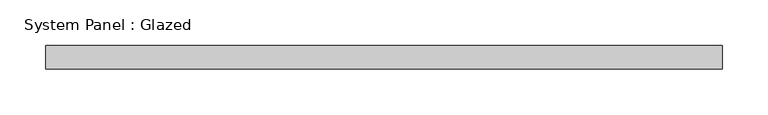
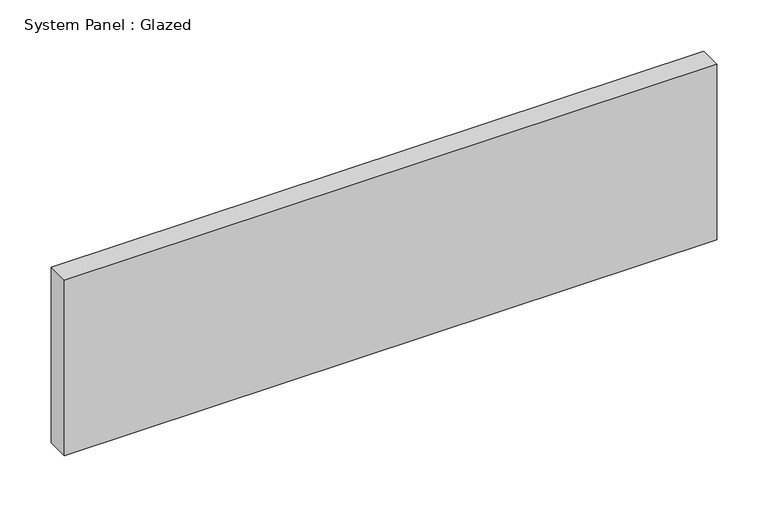
"""IFC4 building model written with IfcOpenShell, lengths in millimetres: plate geometry, System Panel : Glazed."""

from ifc_helpers import new_model, si_unit, origin, origin_with_axes, place, context, project, spatial, polyline, outline, extrude, source, transform, mapped, element, save


def system_panel_glazed_6c905176(model_context):
    return source(origin(), model_context, "Body", "SweptSolid", [
        extrude(outline(polyline([(368.3, 19.05), (-368.3, 19.05), (-368.3, 44.45), (368.3, 44.45), (368.3, 19.05)])), origin_with_axes(), (0.0, 0.0, 1.0), 209.55),
    ])


if __name__ == "__main__":
    model = new_model("IFC4")
    model_context = context("Model", 3, world=origin())
    ifc_project = project(units=[si_unit("LENGTHUNIT", "METRE", prefix="MILLI")], contexts=[model_context])
    site = spatial("IfcSite", under=ifc_project)
    building = spatial("IfcBuilding", under=site)
    placement = place(None, origin())
    system_panel_glazed_shape = system_panel_glazed_6c905176(model_context)
    element("IfcPlate", 1, ObjectType="System Panel : Glazed", at=placement, inside=building, context=model_context, shape_type="MappedRepresentation", body=[
        mapped(system_panel_glazed_shape, transform((0.0, 0.0, 0.0), x_axis=(1.0, 0.0, 0.0), y_axis=(0.0, 1.0, 0.0), z_axis=(0.0, 0.0, 1.0))),
    ])
    save(model, "model.ifc")

# Revit data of these elements
# Type "System Panel : Glazed"
#   Construction Type Id = "GSP4R"
#   Analytic Construction = "1/8 in Pilkington single glazing"
#   Visual Light Transmittance = 0.9
#   Solar Heat Gain Coefficient = 0.86
#   Heat Transfer Coefficient (U) = 1.18115 BTU/(h·ft²·°F)
#   Define Thermal Properties by = 1
# Element 1 (IfcPlate, "System Panel : Glazed")
#   Materials on its faces: "Glass"
# Materials
#   "Glass": class "Glass", colour RGB 0 128 192, transparency 0.75, Description = "Soda Lime Glass", Cost = 0
